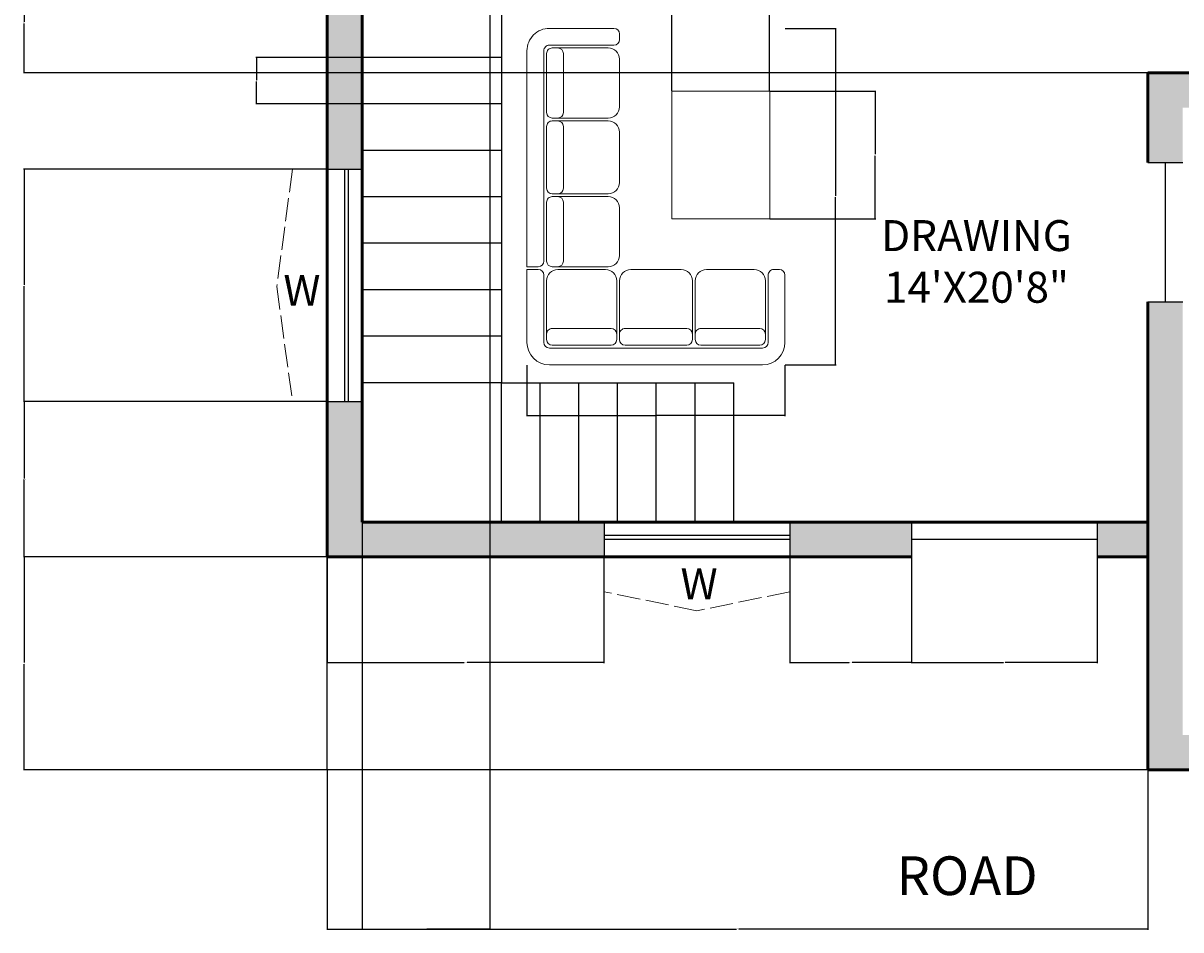
# Model space of a CAD drawing. Units: inches. Extents: x -75 to 416, y -487 to 70.
# Tile 1 of 5: x -75 to 224, y -487 to -253. Entities that reach past the tile are written whole.
import ezdxf

# ---------------------------------------------------------------- set-up
doc = ezdxf.new("R2010")
doc.units = ezdxf.units.IN
doc.header["$MEASUREMENT"] = 0
doc.linetypes.add('ACAD_ISO02W100', pattern=[15, 12, -3])
for name, color, linetype, lineweight in [('A-ANNO-DIMS', 2, 'Continuous', 18), ('A-ANNO-TEXT', 7, 'Continuous', 18), ('A-AREA-IDEN', 7, 'Continuous', 25), ('A-DOOR', 3, 'Continuous', 25), ('A-FLOR-STRS', 7, 'Continuous', 25), ('A-FURN', 8, 'Continuous', 18), ('A-GLAZ', 4, 'Continuous', 25), ('A-GLAZ-OVHD', 4, 'ACAD_ISO02W100', 13), ('A-WALL', 7, 'Continuous', 50), ('A-WALL-PATT', 252, 'Continuous', 13), ('C-PROP', 7, 'Continuous', 25)]:
    doc.layers.add(name, color=color, linetype=linetype, lineweight=lineweight)
doc.styles.get("Standard").update_dxf_attribs({"font": 'arial.ttf'})
doc.dimstyles.get("Standard").update_dxf_attribs({"dimtxt": 0.18, "dimasz": 0.18, "dimexe": 0.18, "dimexo": 0.0625, "dimgap": 0.09, "dimtad": 0, "dimtih": 1, "dimtoh": 1, "dimdec": 4, "dimzin": 0, "dimdsep": 46, "dimtxsty": 'Standard', "dimcen": 0.09, "dimadec": 0, "dimazin": 0, "dimtfac": 1, "dimtdec": 4, "dimtofl": 0, "dimtmove": 0, "dimatfit": 3, "dimfxl": 1, "dimtolj": 1, "dimtzin": 0, "dimarcsym": 0})

# ---------------------------------------------------------------- blocks, each defined once
blk = doc.blocks.new('A$C2AFA021D')
for p, q in [((0.8, 2.3), (0.2, 2.3)), ((0.85, 2.2), (0.85, 2.25)), ((0, 2.1), (0, 0.2)), ((0.15, 0.2), (0.15, 2.1)), ((0.175, 1.55), (0.175, 2.075)), ((0.2, 2.15), (0.8, 2.15)), ((0.225, 2.125), (0.275, 2.125)), ((0.75, 2.125), (0.275, 2.125)), ((0.325, 2.075), (0.325, 1.55)), ((0.85, 1.6), (0.85, 2.025)), ((0.275, 1.5), (0.225, 1.5)), ((0.225, 1.475), (0.275, 1.475)), ((0.275, 1.5), (0.75, 1.5)), ((0.75, 1.475), (0.275, 1.475)), ((0.175, 0.875), (0.175, 1.425)), ((0.325, 1.425), (0.325, 0.875)), ((0.85, 0.925), (0.85, 1.375)), ((0.175, 0.225), (0.175, 0.75)), ((0.275, 0.825), (0.225, 0.825)), ((0.225, 0.8), (0.275, 0.8)), ((0.275, 0.825), (0.75, 0.825)), ((0.75, 0.8), (0.275, 0.8)), ((0.325, 0.75), (0.325, 0.225)), ((0.875, 0.275), (0.875, 0.725)), ((0.975, 0.825), (1.4, 0.825)), ((1.5, 0.725), (1.5, 0.275)), ((1.525, 0.275), (1.525, 0.725)), ((1.625, 0.825), (2.075, 0.825)), ((2.175, 0.725), (2.175, 0.275)), ((2.2, 0.275), (2.2, 0.725)), ((2.3, 0.825), (2.725, 0.825)), ((2.825, 0.725), (2.825, 0.275)), ((2.85, 0.2), (2.85, 0.775)), ((2.9, 0.825), (2.95, 0.825)), ((3, 0.775), (3, 0.2)), ((0.85, 0.275), (0.85, 0.7)), ((1.45, 0.325), (0.925, 0.325)), ((2.125, 0.325), (1.575, 0.325)), ((2.775, 0.325), (2.25, 0.325)), ((0.875, 0.275), (0.875, 0.225)), ((1.5, 0.225), (1.5, 0.275)), ((1.525, 0.275), (1.525, 0.225)), ((2.175, 0.225), (2.175, 0.275)), ((2.2, 0.275), (2.2, 0.225)), ((2.825, 0.225), (2.825, 0.275)), ((0.8, 0.15), (0.2, 0.15)), ((0.275, 0.175), (0.225, 0.175)), ((0.275, 0.175), (0.75, 0.175)), ((0.925, 0.175), (1.45, 0.175)), ((0.925, 0.15), (2.8, 0.15)), ((1.575, 0.175), (2.125, 0.175)), ((2.25, 0.175), (2.775, 0.175)), ((0.85, 0), (0.85, 0.1)), ((0.875, 0.1), (0.875, 0)), ((0.2, 0), (0.85, 0)), ((2.8, 0), (0.875, 0))]:
    blk.add_line(p, q)
for centre, radius, start, end in [((0.2, 2.1), 0.2, 90, 180), ((0.8, 2.25), 0.05, 0, 90), ((0.8, 2.2), 0.05, 270, 0), ((0.2, 2.1), 0.05, 90, 180), ((0.225, 2.075), 0.05, 90, 180), ((0.275, 2.075), 0.05, 0, 90), ((0.75, 2.025), 0.1, 0, 90), ((0.225, 1.55), 0.05, 180, 270), ((0.275, 1.55), 0.05, 270, 0), ((0.75, 1.6), 0.1, 270, 0), ((0.225, 1.425), 0.05, 90, 180), ((0.275, 1.425), 0.05, 0, 90), ((0.75, 1.375), 0.1, 360, 90), ((0.225, 0.875), 0.05, 180, 270), ((0.275, 0.875), 0.05, 270, 0), ((0.75, 0.925), 0.1, 270, 0), ((0.225, 0.75), 0.05, 90, 180), ((0.275, 0.75), 0.05, 0, 90), ((0.75, 0.7), 0.1, 0, 90), ((0.975, 0.725), 0.1, 90, 180), ((1.4, 0.725), 0.1, 0, 90), ((1.625, 0.725), 0.1, 90, 180), ((2.075, 0.725), 0.1, 0, 90), ((2.3, 0.725), 0.1, 90, 180), ((2.725, 0.725), 0.1, 0, 90), ((2.9, 0.775), 0.05, 90, 180), ((2.95, 0.775), 0.05, 0, 90), ((0.925, 0.275), 0.05, 90, 180), ((1.45, 0.275), 0.05, 360, 90), ((1.575, 0.275), 0.05, 90, 180), ((2.125, 0.275), 0.05, 360, 90), ((2.25, 0.275), 0.05, 90, 180), ((2.775, 0.275), 0.05, 360, 90), ((0.225, 0.225), 0.05, 180, 270), ((0.275, 0.225), 0.05, 270, 0), ((0.75, 0.275), 0.1, 270, 0), ((0.925, 0.225), 0.05, 180, 270), ((1.45, 0.225), 0.05, 270, 0), ((1.575, 0.225), 0.05, 180, 270), ((2.125, 0.225), 0.05, 270, 0), ((2.25, 0.225), 0.05, 180, 270), ((2.775, 0.225), 0.05, 270, 0), ((0.2, 0.2), 0.2, 180, 270), ((0.2, 0.2), 0.05, 180, 270), ((0.8, 0.1), 0.05, 0, 90), ((0.925, 0.1), 0.05, 90, 180), ((2.8, 0.2), 0.2, 270, 0), ((2.8, 0.2), 0.05, 270, 0)]:
    blk.add_arc(centre, radius, start, end)
blk = doc.blocks.new('WIN-48IN')
for p, q in [((0, 9), (0, 0)), ((48, 9), (48, 0)), ((48, 5.5), (0, 5.5)), ((48, 4.5), (0, 4.5))]:
    blk.add_line(p, q)
blk = doc.blocks.new('WIN-SHADE-48IN')
at = {"ltscale": 0.5}
for p, q in [((0, 4.91), (0, 13.91)), ((48, 13.91), (48, 4.91)), ((24, 0), (0, 4.91)), ((48, 4.91), (24, 0))]:
    blk.add_line(p, q, dxfattribs=at)
blk = doc.blocks.new('DOOR-36IN')
for p, q in [((0, 9), (0, 0)), ((36, 9), (36, 0)), ((36, 4.5), (0, 4.5))]:
    blk.add_line(p, q)
blk = doc.blocks.new('*D32')
at = {"layer": 'A-ANNO-DIMS', "color": 0, "lineweight": -2, "transparency": 16777216}
for p, q in [((121.86, -253.84), (135.01, -253.84)), ((134.83, -254.02), (134.83, -297.13)), ((134.83, -340.6), (134.83, -297.49)), ((121.86, -340.78), (135.01, -340.78))]:
    blk.add_line(p, q, dxfattribs=at)
at = {"layer": 'A-ANNO-DIMS', "color": 0, "transparency": 16777216}
for points in [[(134.8, -254.02), (134.86, -254.02), (134.83, -253.84)], [(134.8, -340.6), (134.86, -340.6), (134.83, -340.78)]]:
    blk.add_solid(points, dxfattribs=at)
at = {"layer": 'Defpoints', "color": 0, "transparency": 16777216}
for p in [(121.79, -253.84), (134.83, -253.84), (121.79, -340.78)]:
    blk.add_point(p, dxfattribs=at)
at = {"layer": 'A-ANNO-DIMS', "color": 0, "transparency": 16777216, "insert": (134.83, -297.31), "char_height": 0.18, "attachment_point": 5}
blk.add_mtext('\\A1;SOFA 87', dxfattribs=at)
blk = doc.blocks.new('*D33')
at = {"layer": 'A-ANNO-DIMS', "color": 0, "lineweight": -2, "transparency": 16777216}
for p, q in [((55.14, -340.84), (55.14, -354)), ((121.79, -340.84), (121.79, -354)), ((55.32, -353.82), (88.25, -353.82)), ((121.61, -353.82), (88.69, -353.82))]:
    blk.add_line(p, q, dxfattribs=at)
at = {"layer": 'A-ANNO-DIMS', "color": 0, "transparency": 16777216}
for points in [[(55.32, -353.79), (55.32, -353.85), (55.14, -353.82)], [(121.61, -353.79), (121.61, -353.85), (121.79, -353.82)]]:
    blk.add_solid(points, dxfattribs=at)
at = {"layer": 'Defpoints', "color": 0, "transparency": 16777216}
for p in [(55.14, -340.78), (121.79, -340.78), (121.79, -353.82)]:
    blk.add_point(p, dxfattribs=at)
at = {"layer": 'A-ANNO-DIMS', "color": 0, "transparency": 16777216, "insert": (88.47, -353.82), "char_height": 0.18, "attachment_point": 5}
blk.add_mtext('\\A1;67', dxfattribs=at)
blk = doc.blocks.new('*D36')
at = {"layer": 'A-ANNO-DIMS', "color": 0, "lineweight": -2, "transparency": 16777216}
for p, q in [((3.55, -445.44), (3.55, -486.72)), ((215.55, -445.44), (215.55, -486.72)), ((3.73, -486.54), (109.26, -486.54)), ((215.37, -486.54), (109.84, -486.54))]:
    blk.add_line(p, q, dxfattribs=at)
at = {"layer": 'A-ANNO-DIMS', "color": 0, "transparency": 16777216}
for points in [[(3.73, -486.51), (3.73, -486.57), (3.55, -486.54)], [(215.37, -486.51), (215.37, -486.57), (215.55, -486.54)]]:
    blk.add_solid(points, dxfattribs=at)
at = {"layer": 'Defpoints', "color": 0, "transparency": 16777216}
for p in [(3.55, -445.37), (215.55, -445.37), (215.55, -486.54)]:
    blk.add_point(p, dxfattribs=at)
at = {"layer": 'A-ANNO-DIMS', "color": 0, "transparency": 16777216, "insert": (109.55, -486.54), "char_height": 0.18, "attachment_point": 5}
blk.add_mtext('\\A1;212', dxfattribs=at)
blk = doc.blocks.new('*D37')
at = {"layer": 'A-ANNO-DIMS', "color": 0, "lineweight": -2, "transparency": 16777216}
for p, q in [((3.49, -390.37), (-74.89, -390.37)), ((-74.71, -390.55), (-74.71, -417.69)), ((-74.71, -445.19), (-74.71, -418.06)), ((3.49, -445.37), (-74.89, -445.37))]:
    blk.add_line(p, q, dxfattribs=at)
at = {"layer": 'A-ANNO-DIMS', "color": 0, "transparency": 16777216}
for points in [[(-74.74, -390.55), (-74.68, -390.55), (-74.71, -390.37)], [(-74.74, -445.19), (-74.68, -445.19), (-74.71, -445.37)]]:
    blk.add_solid(points, dxfattribs=at)
at = {"layer": 'Defpoints', "color": 0, "transparency": 16777216}
for p in [(-74.71, -390.37), (3.55, -390.37), (3.55, -445.37)]:
    blk.add_point(p, dxfattribs=at)
at = {"layer": 'A-ANNO-DIMS', "color": 0, "transparency": 16777216, "insert": (-74.71, -417.87), "char_height": 0.18, "attachment_point": 5}
blk.add_mtext('\\A1;55', dxfattribs=at)
blk = doc.blocks.new('*D46')
at = {"layer": 'A-ANNO-DIMS', "color": 0, "lineweight": -2, "transparency": 16777216}
for p, q in [((3.49, -290.25), (-74.89, -290.25)), ((-74.71, -290.43), (-74.71, -320.07)), ((-74.71, -350.07), (-74.71, -320.43)), ((3.49, -350.25), (-74.89, -350.25))]:
    blk.add_line(p, q, dxfattribs=at)
at = {"layer": 'A-ANNO-DIMS', "color": 0, "transparency": 16777216}
for points in [[(-74.74, -290.43), (-74.68, -290.43), (-74.71, -290.25)], [(-74.74, -350.07), (-74.68, -350.07), (-74.71, -350.25)]]:
    blk.add_solid(points, dxfattribs=at)
at = {"layer": 'Defpoints', "color": 0, "transparency": 16777216}
for p in [(3.55, -290.25), (-74.71, -350.25), (3.55, -350.25)]:
    blk.add_point(p, dxfattribs=at)
at = {"layer": 'A-ANNO-DIMS', "color": 0, "transparency": 16777216, "insert": (-74.71, -320.25), "char_height": 0.18, "attachment_point": 5}
blk.add_mtext('\\A1;60', dxfattribs=at)
blk = doc.blocks.new('*D47')
at = {"layer": 'A-ANNO-DIMS', "color": 0, "lineweight": -2, "transparency": 16777216}
for p, q in [((3.49, -350.25), (-74.89, -350.25)), ((-74.71, -350.43), (-74.71, -370.13)), ((-74.71, -390.19), (-74.71, -370.49)), ((3.49, -390.37), (-74.89, -390.37))]:
    blk.add_line(p, q, dxfattribs=at)
at = {"layer": 'A-ANNO-DIMS', "color": 0, "transparency": 16777216}
for points in [[(-74.74, -350.43), (-74.68, -350.43), (-74.71, -350.25)], [(-74.74, -390.19), (-74.68, -390.19), (-74.71, -390.37)]]:
    blk.add_solid(points, dxfattribs=at)
at = {"layer": 'Defpoints', "color": 0, "transparency": 16777216}
for p in [(3.55, -350.25), (-74.71, -390.37), (3.55, -390.37)]:
    blk.add_point(p, dxfattribs=at)
at = {"layer": 'A-ANNO-DIMS', "color": 0, "transparency": 16777216, "insert": (-74.71, -370.31), "char_height": 0.18, "attachment_point": 5}
blk.add_mtext('\\A1;40.13', dxfattribs=at)
blk = doc.blocks.new('*D48')
at = {"layer": 'A-ANNO-DIMS', "color": 0, "lineweight": -2, "transparency": 16777216}
for p, q in [((3.55, -390.44), (3.55, -417.81)), ((75.04, -390.44), (75.04, -417.81)), ((3.73, -417.63), (38.9, -417.63)), ((74.86, -417.63), (39.69, -417.63))]:
    blk.add_line(p, q, dxfattribs=at)
at = {"layer": 'A-ANNO-DIMS', "color": 0, "transparency": 16777216}
for points in [[(3.73, -417.6), (3.73, -417.66), (3.55, -417.63)], [(74.86, -417.6), (74.86, -417.66), (75.04, -417.63)]]:
    blk.add_solid(points, dxfattribs=at)
at = {"layer": 'Defpoints', "color": 0, "transparency": 16777216}
for p in [(3.55, -390.37), (75.04, -390.37), (3.55, -417.63)]:
    blk.add_point(p, dxfattribs=at)
at = {"layer": 'A-ANNO-DIMS', "color": 0, "transparency": 16777216, "insert": (39.3, -417.63), "char_height": 0.18, "attachment_point": 5}
blk.add_mtext('\\A1;71.49', dxfattribs=at)
blk = doc.blocks.new('*D49')
at = {"layer": 'A-ANNO-DIMS', "color": 0, "lineweight": -2, "transparency": 16777216}
for p, q in [((123.04, -390.44), (123.04, -417.81)), ((154.45, -390.44), (154.45, -417.81)), ((123.22, -417.63), (138.37, -417.63)), ((154.27, -417.63), (139.12, -417.63))]:
    blk.add_line(p, q, dxfattribs=at)
at = {"layer": 'A-ANNO-DIMS', "color": 0, "transparency": 16777216}
for points in [[(123.22, -417.6), (123.22, -417.66), (123.04, -417.63)], [(154.27, -417.6), (154.27, -417.66), (154.45, -417.63)]]:
    blk.add_solid(points, dxfattribs=at)
at = {"layer": 'Defpoints', "color": 0, "transparency": 16777216}
for p in [(123.04, -390.37), (154.45, -390.37), (123.04, -417.63)]:
    blk.add_point(p, dxfattribs=at)
at = {"layer": 'A-ANNO-DIMS', "color": 0, "transparency": 16777216, "insert": (138.75, -417.63), "char_height": 0.18, "attachment_point": 5}
blk.add_mtext('\\A1;31.41', dxfattribs=at)
blk = doc.blocks.new('*D50')
at = {"layer": 'A-ANNO-DIMS', "color": 0, "lineweight": -2, "transparency": 16777216}
for p, q in [((154.45, -390.44), (154.45, -417.81)), ((202.45, -390.44), (202.45, -417.81)), ((154.63, -417.63), (178.23, -417.63)), ((202.27, -417.63), (178.68, -417.63))]:
    blk.add_line(p, q, dxfattribs=at)
at = {"layer": 'A-ANNO-DIMS', "color": 0, "transparency": 16777216}
for points in [[(154.63, -417.6), (154.63, -417.66), (154.45, -417.63)], [(202.27, -417.6), (202.27, -417.66), (202.45, -417.63)]]:
    blk.add_solid(points, dxfattribs=at)
at = {"layer": 'Defpoints', "color": 0, "transparency": 16777216}
for p in [(154.45, -390.37), (202.45, -390.37), (154.45, -417.63)]:
    blk.add_point(p, dxfattribs=at)
at = {"layer": 'A-ANNO-DIMS', "color": 0, "transparency": 16777216, "insert": (178.45, -417.63), "char_height": 0.18, "attachment_point": 5}
blk.add_mtext('\\A1;48', dxfattribs=at)
blk = doc.blocks.new('*D55')
at = {"layer": 'A-ANNO-DIMS', "color": 0, "lineweight": -2, "transparency": 16777216}
for p, q in [((269.49, -239.36), (-74.89, -239.36)), ((-74.71, -239.54), (-74.71, -252.19)), ((-74.71, -265.19), (-74.71, -252.55)), ((269.49, -265.37), (-74.89, -265.37))]:
    blk.add_line(p, q, dxfattribs=at)
at = {"layer": 'A-ANNO-DIMS', "color": 0, "transparency": 16777216}
for points in [[(-74.74, -239.54), (-74.68, -239.54), (-74.71, -239.36)], [(-74.74, -265.19), (-74.68, -265.19), (-74.71, -265.37)]]:
    blk.add_solid(points, dxfattribs=at)
at = {"layer": 'Defpoints', "color": 0, "transparency": 16777216}
for p in [(269.55, -239.36), (-74.71, -265.37), (269.55, -265.37)]:
    blk.add_point(p, dxfattribs=at)
at = {"layer": 'A-ANNO-DIMS', "color": 0, "transparency": 16777216, "insert": (-74.71, -252.37), "char_height": 0.18, "attachment_point": 5}
blk.add_mtext('\\A1;26.01', dxfattribs=at)
blk = doc.blocks.new('*D63')
at = {"layer": 'A-ANNO-DIMS', "color": 0, "lineweight": -2, "transparency": 16777216}
for p, q in [((12.49, -261.37), (-14.89, -261.37)), ((-14.71, -261.55), (-14.71, -267.19)), ((-14.71, -273.19), (-14.71, -267.55)), ((12.49, -273.37), (-14.89, -273.37))]:
    blk.add_line(p, q, dxfattribs=at)
at = {"layer": 'A-ANNO-DIMS', "color": 0, "transparency": 16777216}
for points in [[(-14.74, -261.55), (-14.68, -261.55), (-14.71, -261.37)], [(-14.74, -273.19), (-14.68, -273.19), (-14.71, -273.37)]]:
    blk.add_solid(points, dxfattribs=at)
at = {"layer": 'Defpoints', "color": 0, "transparency": 16777216}
for p in [(-14.71, -261.37), (12.55, -261.37), (12.55, -273.37)]:
    blk.add_point(p, dxfattribs=at)
at = {"layer": 'A-ANNO-DIMS', "color": 0, "transparency": 16777216, "insert": (-14.71, -267.37), "char_height": 0.18, "attachment_point": 5}
blk.add_mtext('\\A1;12', dxfattribs=at)
blk = doc.blocks.new('*D64')
at = {"layer": 'A-ANNO-DIMS', "color": 0, "lineweight": -2, "transparency": 16777216}
for p, q in [((92.6, -270.01), (92.6, -242.63)), ((92.78, -242.81), (104.83, -242.81)), ((117.66, -242.81), (105.62, -242.81)), ((117.84, -270.01), (117.84, -242.63))]:
    blk.add_line(p, q, dxfattribs=at)
at = {"layer": 'A-ANNO-DIMS', "color": 0, "transparency": 16777216}
for points in [[(92.78, -242.78), (92.78, -242.84), (92.6, -242.81)], [(117.66, -242.78), (117.66, -242.84), (117.84, -242.81)]]:
    blk.add_solid(points, dxfattribs=at)
at = {"layer": 'Defpoints', "color": 0, "transparency": 16777216}
for p in [(117.84, -242.81), (92.6, -270.07), (117.84, -270.07)]:
    blk.add_point(p, dxfattribs=at)
at = {"layer": 'A-ANNO-DIMS', "color": 0, "transparency": 16777216, "insert": (105.22, -242.81), "char_height": 0.18, "attachment_point": 5}
blk.add_mtext('\\A1;25.24', dxfattribs=at)
blk = doc.blocks.new('*D65')
at = {"layer": 'A-ANNO-DIMS', "color": 0, "lineweight": -2, "transparency": 16777216}
for p, q in [((117.9, -270.07), (145.28, -270.07)), ((145.1, -270.25), (145.1, -286.38)), ((145.1, -302.88), (145.1, -286.75)), ((117.9, -303.06), (145.28, -303.06))]:
    blk.add_line(p, q, dxfattribs=at)
at = {"layer": 'A-ANNO-DIMS', "color": 0, "transparency": 16777216}
for points in [[(145.07, -270.25), (145.13, -270.25), (145.1, -270.07)], [(145.07, -302.88), (145.13, -302.88), (145.1, -303.06)]]:
    blk.add_solid(points, dxfattribs=at)
at = {"layer": 'Defpoints', "color": 0, "transparency": 16777216}
for p in [(117.84, -270.07), (117.84, -303.06), (145.1, -303.06)]:
    blk.add_point(p, dxfattribs=at)
at = {"layer": 'A-ANNO-DIMS', "color": 0, "transparency": 16777216, "insert": (145.1, -286.57), "char_height": 0.18, "attachment_point": 5}
blk.add_mtext('\\A1;32.99', dxfattribs=at)
blk = doc.blocks.new('*D70')
at = {"layer": 'A-ANNO-DIMS', "color": 0, "lineweight": -2, "transparency": 16777216}
for p, q in [((45.55, -168.31), (45.55, -486.72)), ((12.55, -178.81), (12.55, -486.72)), ((12.73, -486.54), (28.83, -486.54)), ((45.37, -486.54), (29.27, -486.54))]:
    blk.add_line(p, q, dxfattribs=at)
at = {"layer": 'A-ANNO-DIMS', "color": 0, "transparency": 16777216}
for points in [[(12.73, -486.51), (12.73, -486.57), (12.55, -486.54)], [(45.37, -486.51), (45.37, -486.57), (45.55, -486.54)]]:
    blk.add_solid(points, dxfattribs=at)
at = {"layer": 'Defpoints', "color": 0, "transparency": 16777216}
for p in [(45.55, -168.25), (12.55, -178.75), (45.55, -486.54)]:
    blk.add_point(p, dxfattribs=at)
at = {"layer": 'A-ANNO-DIMS', "color": 0, "transparency": 16777216, "insert": (29.05, -486.54), "char_height": 0.18, "attachment_point": 5}
blk.add_mtext('\\A1;33', dxfattribs=at)

msp = doc.modelspace()

# ---------------------------------------------------------------- hatches: boundary and pattern name
at = {"layer": 'A-WALL-PATT'}
h = msp.add_hatch(color=256, dxfattribs=at)
h.dxf.hatch_style = 1
h.paths.add_polyline_path([(84.8603, 28.6255), (3.5531, 28.6255), (3.5531, -23.8141), (12.5531, -23.8141), (12.5531, 19.6255), (84.8603, 19.6255)])
h.paths.add_polyline_path([(263.7442, 28.6255), (132.8603, 28.6255), (132.8603, 19.6255), (146.5531, 19.6255), (180.5531, 19.6255), (180.5531, -124.3745), (180.5531, -133.3745), (200.467, -133.3745), (200.467, -124.3745), (189.5531, -124.3745), (189.5531, 19.6255), (263.7442, 19.6255)])
h.paths.add_polyline_path([(374.5531, 28.6255), (311.7442, 28.6255), (311.7442, 19.6255), (327.5531, 19.6255), (365.5531, 19.6255), (365.5531, -37.0191), (374.5531, -37.0191)])
h.paths.add_polyline_path([(144.5531, -124.3745), (12.5531, -124.3745), (12.5531, -71.8141), (3.5531, -71.8141), (3.5531, -148.6403), (12.5531, -148.6403), (12.5531, -133.3745), (144.5531, -133.3745)])
h.paths.add_polyline_path([(117.5531, -133.3745), (108.5531, -133.3745), (108.5531, -161.7866), (117.5531, -161.7866)])
h.paths.add_polyline_path([(374.5531, -85.0191), (365.5531, -85.0191), (365.5531, -124.3745), (236.467, -124.3745), (236.467, -133.3745), (374.5531, -133.3745)])
h.paths.add_polyline_path([(374.5531, -133.3745), (365.5531, -133.3745), (365.5531, -183.1692), (374.5531, -183.1692)])
h.paths.add_polyline_path([(374.5531, -231.1692), (365.5531, -231.1692), (365.5531, -265.3745), (260.5531, -265.3745), (260.5531, -274.3745), (374.5531, -274.3745)])
h.paths.add_polyline_path([(260.5531, -265.3745), (215.5531, -265.3745), (215.5531, -288.4908), (224.5531, -288.4908), (224.5531, -274.3745), (260.5531, -274.3745)])
h.paths.add_polyline_path([(374.5531, -274.3745), (365.5531, -274.3745), (365.5531, -345.9302), (374.5531, -345.9302)])
h.paths.add_polyline_path([(374.5531, -393.9302), (365.5531, -393.9302), (365.5531, -436.3745), (321.1982, -436.3745), (321.1982, -445.3745), (374.5531, -445.3745)])
h.paths.add_polyline_path([(224.5531, -324.4908), (215.5531, -324.4908), (215.5531, -445.3745), (273.1982, -445.3745), (273.1982, -436.3745), (265.0531, -436.3745), (245.0531, -436.3745), (224.5531, -436.3745)])
h.paths.add_polyline_path([(12.5531, -183.233), (3.5531, -183.233), (3.5531, -214.3745), (117.5531, -214.3745), (117.5531, -197.7866), (108.5531, -197.7866), (108.5531, -205.3745), (12.5531, -205.3745)])
h.paths.add_polyline_path([(12.5531, -214.3745), (3.5531, -214.3745), (3.5531, -290.2477), (12.5531, -290.2477)])
h.paths.add_polyline_path([(75.0426, -381.3745), (12.5531, -381.3745), (12.5531, -350.2477), (3.5531, -350.2477), (3.5531, -390.3745), (75.0426, -390.3745)])
h.paths.add_polyline_path([(154.4537, -381.3745), (123.0426, -381.3745), (123.0426, -390.3745), (154.4537, -390.3745)])
h.paths.add_polyline_path([(215.5531, -381.3745), (202.4537, -381.3745), (202.4537, -390.3745), (215.5531, -390.3745)])

# ---------------------------------------------------------------- linework, layer by layer
at = {"layer": 'A-DOOR'}
for p, q in [((154.4537, -381.3745), (154.4537, -390.3745)), ((202.4537, -381.3745), (202.4537, -390.3745)), ((202.4537, -385.8745), (154.4537, -385.8745))]:
    msp.add_line(p, q, dxfattribs=at)
at = {"layer": 'A-FLOR-STRS'}
for p, q in [((48.5531, -250.3745), (48.5531, -345.3745)), ((48.5531, -261.3745), (12.5531, -261.3745)), ((48.5531, -273.3745), (12.5531, -273.3745)), ((48.5531, -285.3745), (12.5531, -285.3745)), ((48.5531, -297.3745), (12.5531, -297.3745)), ((48.5531, -309.3745), (12.5531, -309.3745)), ((48.5531, -321.3745), (12.5531, -321.3745)), ((48.5531, -333.3745), (12.5531, -333.3745)), ((48.5531, -345.3745), (12.5531, -345.3745)), ((48.5531, -381.3745), (48.5531, -345.3745)), ((48.5531, -345.3745), (108.5531, -345.3745)), ((58.5531, -381.3745), (58.5531, -345.3745)), ((68.5531, -381.3745), (68.5531, -345.3745)), ((78.5531, -381.3745), (78.5531, -345.3745)), ((88.5531, -381.3745), (88.5531, -345.3745)), ((98.5531, -381.3745), (98.5531, -345.3745)), ((108.5531, -381.3745), (108.5531, -345.3745))]:
    msp.add_line(p, q, dxfattribs=at)
at = {"layer": 'A-FURN'}
msp.add_lwpolyline([(92.6027, -270.0727), (117.8408, -270.0727), (117.8408, -303.0598), (92.6027, -303.0598)], close=True, dxfattribs=at)
at = {"layer": 'A-GLAZ'}
for p, q in [((3.5531, -290.2477), (12.5531, -290.2477)), ((8.0531, -350.2477), (8.0531, -290.2477)), ((9.0531, -350.2477), (9.0531, -290.2477)), ((3.5531, -350.2477), (12.5531, -350.2477))]:
    msp.add_line(p, q, dxfattribs=at)
at = {"layer": 'A-GLAZ-OVHD', "ltscale": 0.5}
for p, q in [((-5.4469, -290.2477), (-9.4958, -320.5597)), ((3.5531, -290.2477), (-5.4469, -290.2477)), ((-9.4958, -320.5597), (-5.4469, -350.2477)), ((-5.4469, -350.2477), (3.5531, -350.2477))]:
    msp.add_line(p, q, dxfattribs=at)
at = {"layer": 'A-WALL'}
for p, q in [((3.5531, 28.6255), (3.5531, -390.3745)), ((12.5531, -214.3745), (12.5531, -381.3745)), ((215.5531, -265.3745), (365.5531, -265.3745)), ((215.5531, -265.3745), (215.5531, -288.4908)), ((215.5531, -324.4908), (215.5531, -445.3745)), ((12.5531, -381.3745), (215.5531, -381.3745)), ((3.5531, -390.3745), (154.4537, -390.3745)), ((202.4537, -390.3745), (215.5531, -390.3745)), ((215.5531, -445.3745), (374.5531, -445.3745))]:
    msp.add_line(p, q, dxfattribs=at)
at = {"layer": 'C-PROP'}
for p, q in [((3.5531, -445.3745), (3.5531, -390.3745)), ((215.5531, -445.3745), (3.5531, -445.3745))]:
    msp.add_line(p, q, dxfattribs=at)

# ---------------------------------------------------------------- block references
at = {"layer": 'A-DOOR', "rotation": 89.99999999999999}
msp.add_blockref('DOOR-36IN', (224.5526, -324.4909), dxfattribs=at)
at = {"layer": 'A-FURN', "xscale": -28.97905733467954, "yscale": 28.97905733467954, "zscale": 28.97905733467954, "rotation": 270}
msp.add_blockref('A$C2AFA021D', (55.141, -340.7803), dxfattribs=at)
at = {"layer": 'A-GLAZ'}
msp.add_blockref('WIN-48IN', (75.043, -390.374), dxfattribs=at)
at = {"layer": 'A-GLAZ-OVHD'}
msp.add_blockref('WIN-SHADE-48IN', (75.0423, -404.284), dxfattribs=at)

# ---------------------------------------------------------------- texts
at = {"layer": 'A-ANNO-TEXT', "attachment_point": 1}
for s, width, insert, char_height in [('\\pxqc;W', 15.130285, (-10.562, -317.5199), 8), ('\\pxqc;W', 15.130285, (92.0446, -393.3452), 8), ('\\pxqc;{\\fArial|b1|i0|c0|p34;ROAD}', 144.357858, (96.6637, -467.7412), 10)]:
    msp.add_mtext_dynamic_manual_height_columns(s, width=width, gutter_width=1, heights=[0], dxfattribs=dict(at, insert=insert, char_height=char_height))
at = {"layer": 'A-AREA-IDEN', "insert": (99.0938, -303.3856), "char_height": 8, "attachment_point": 1}
msp.add_mtext_dynamic_manual_height_columns('\\pxqc;DRAWING\\P14\'X20\'8"', width=144.357858, gutter_width=1, heights=[0], dxfattribs=at)

# ---------------------------------------------------------------- dimensions: what is measured, and where the dimension line sits
at = {"layer": 'A-ANNO-DIMS'}
for base, p1, p2, override, picture, middle in [((45.553, -486.5442), (12.5531, -178.7524), (45.553, -168.2524), {"dimdec": 0, "dimlfac": 1, "dimrnd": 0, "dimzin": 0, "dimdsep": 46, "dimlunit": 2}, '*D70', (29.053, -486.5442)), ((117.8408, -242.8127), (92.6027, -270.0727), (117.8408, -270.0727), {"dimdec": 2, "dimlfac": 1, "dimrnd": 0, "dimzin": 0, "dimdsep": 46, "dimlunit": 2}, '*D64', (105.2218, -242.8127)), ((121.7928, -353.8208), (55.141, -340.7803), (121.7928, -340.7803), {"dimdec": 0, "dimlfac": 1, "dimrnd": 0, "dimzin": 0, "dimdsep": 46, "dimlunit": 2}, '*D33', (88.4669, -353.8208)), ((215.5531, -486.5442), (3.5531, -445.3745), (215.5531, -445.3745), {"dimdec": 0, "dimlfac": 1, "dimrnd": 0, "dimzin": 0, "dimdsep": 46, "dimlunit": 2}, '*D36', (109.5531, -486.5442))]:
    dim = msp.add_linear_dim(base=base, p1=p1, p2=p2, dimstyle='Standard', override=override, dxfattribs=at)
    dim.commit()
    dim.dimension.update_dxf_attribs({"geometry": picture, "text_midpoint": middle})
for base, p1, p2, angle, override, picture, middle in [((-74.7069, -265.3745), (269.5531, -239.362), (269.5531, -265.3745), 90, {"dimdec": 2, "dimlfac": 1, "dimrnd": 0, "dimzin": 0, "dimdsep": 46, "dimlunit": 2}, '*D55', (-74.7069, -252.3682)), ((-14.7069, -261.3745), (12.5531, -273.3745), (12.5531, -261.3745), 90, {"dimdec": 0, "dimlfac": 1, "dimrnd": 0, "dimzin": 0, "dimdsep": 46, "dimlunit": 2}, '*D63', (-14.7069, -267.3745)), ((145.1008, -303.0598), (117.8408, -270.0727), (117.8408, -303.0598), 270, {"dimdec": 2, "dimlfac": 1, "dimrnd": 0, "dimzin": 0, "dimdsep": 46, "dimlunit": 2}, '*D65', (145.1008, -286.5663)), ((-74.7069, -350.2477), (3.5531, -290.2477), (3.5531, -350.2477), 90, {"dimdec": 0, "dimlfac": 1, "dimrnd": 0, "dimzin": 0, "dimdsep": 46, "dimlunit": 2}, '*D46', (-74.7069, -320.2477)), ((-74.7069, -390.3745), (3.5531, -350.2477), (3.5531, -390.3745), 90, {"dimdec": 2, "dimlfac": 1, "dimrnd": 0, "dimzin": 0, "dimdsep": 46, "dimlunit": 2}, '*D47', (-74.7069, -370.3111)), ((-74.7069, -390.3745), (3.5531, -445.3745), (3.5531, -390.3745), 90, {"dimdec": 0, "dimlfac": 1, "dimrnd": 0, "dimzin": 0, "dimdsep": 46, "dimlunit": 2}, '*D37', (-74.7069, -417.8745)), ((3.5531, -417.6345), (75.0426, -390.3745), (3.5531, -390.3745), 180, {"dimdec": 2, "dimlfac": 1, "dimrnd": 0, "dimzin": 0, "dimdsep": 46, "dimlunit": 2}, '*D48', (39.2978, -417.6345)), ((123.0426, -417.6345), (154.4537, -390.3745), (123.0426, -390.3745), 180, {"dimdec": 2, "dimlfac": 1, "dimrnd": 0, "dimzin": 0, "dimdsep": 46, "dimlunit": 2}, '*D49', (138.7481, -417.6345)), ((154.4537, -417.6345), (202.4537, -390.3745), (154.4537, -390.3745), 180, {"dimdec": 0, "dimlfac": 1, "dimrnd": 0, "dimzin": 0, "dimdsep": 46, "dimlunit": 2}, '*D50', (178.4537, -417.6345))]:
    dim = msp.add_linear_dim(base=base, p1=p1, p2=p2, angle=angle, dimstyle='Standard', override=override, dxfattribs=at)
    dim.commit()
    dim.dimension.update_dxf_attribs({"geometry": picture, "text_midpoint": middle})
dim = msp.add_linear_dim(base=(134.8334, -253.8431), p1=(121.7928, -340.7803), p2=(121.7928, -253.8431), angle=90, text='SOFA <>', dimstyle='Standard', override={"dimdec": 0, "dimlfac": 1, "dimrnd": 0, "dimzin": 0, "dimdsep": 46, "dimlunit": 2}, dxfattribs=at)
dim.commit()
dim.dimension.update_dxf_attribs({"geometry": '*D32', "text_midpoint": (134.8334, -297.3117)})

doc.saveas('drawing.dxf')
